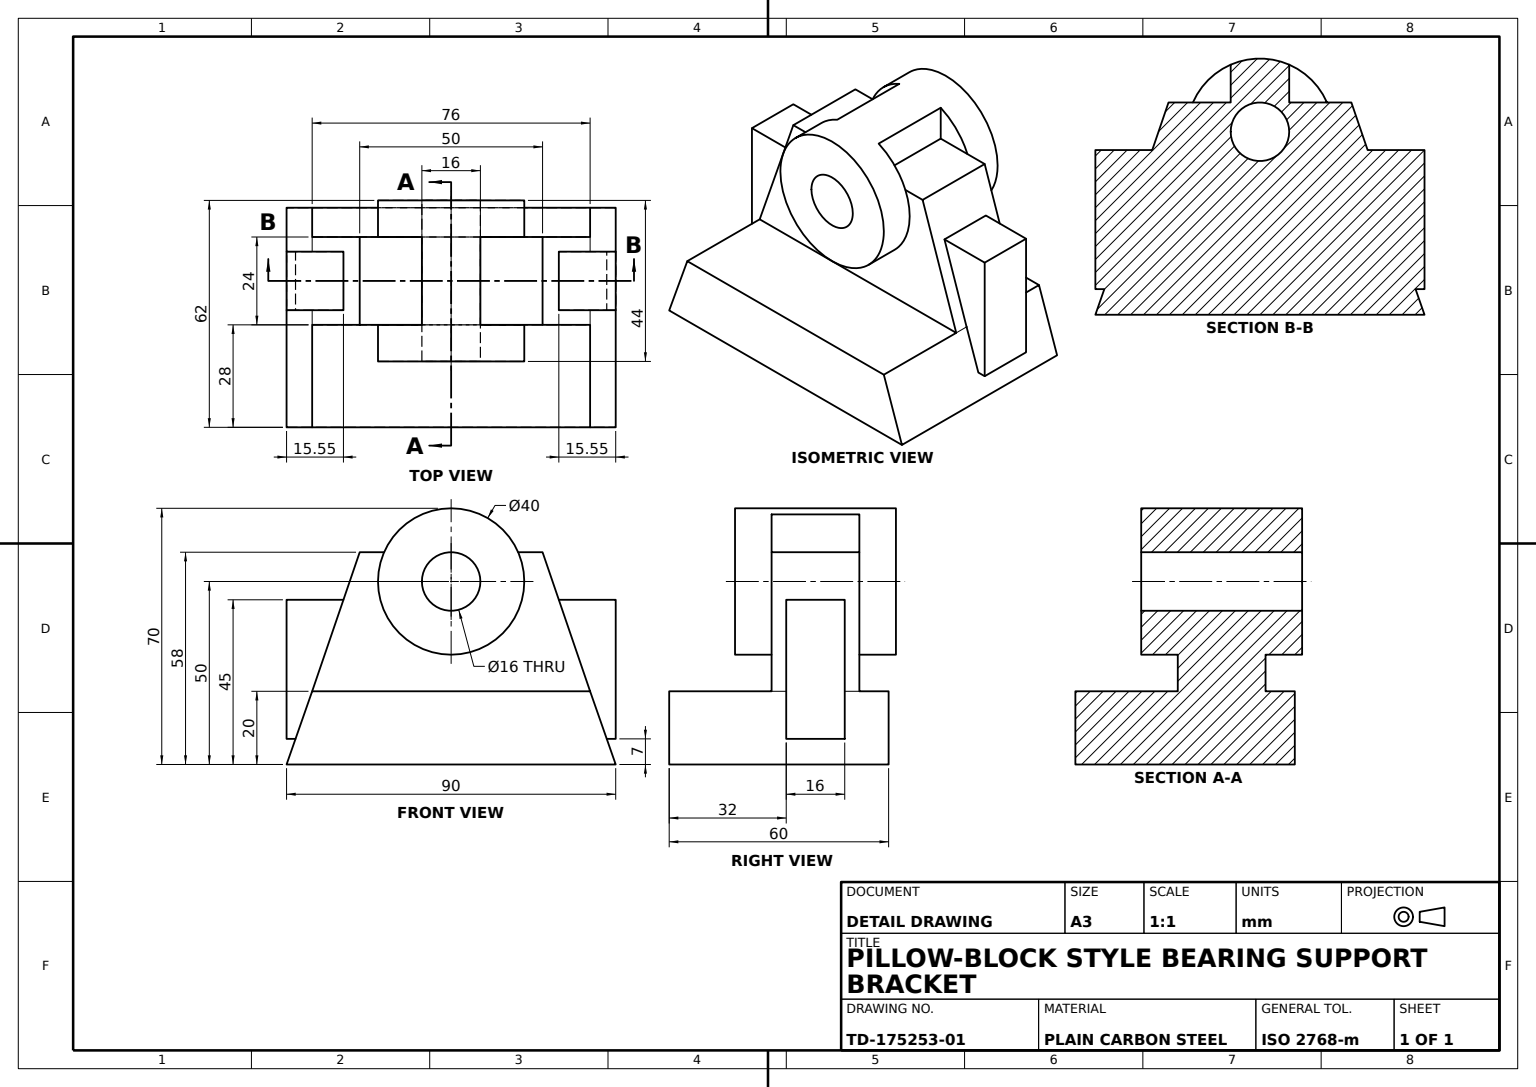
from build123d import *

# Parameters (mm, degrees)
BASE_BLOCK_DEPTH      = 20
BASE_RECESS_CUT_DEPTH = 75
HUB_CIRCLE_SKETCH_R   = 20
BEARING_HUB_DEPTH     = 44
SUPPORT_WEB_DEPTH     = 24
SIDE_WINDOW_CUT_DEPTH = 24
BEARING_BORE_SKETCH_R = 8
BEARING_BORE_DEPTH    = 57
SIDE_RIB_DEPTH        = 20


with BuildPart() as part:
    # Base Profile Sketch → Base Block (new body)
    with BuildSketch(Plane(origin=(0, 0, 0), x_dir=(1, 0, 0), z_dir=(0, 1, 0))):
        Polygon((30, 0), (30, 45), (-30, 45), (-30, -45), (30, -45), align=None)
    extrude(amount=BASE_BLOCK_DEPTH)

    # Base Recess Sketch → Base Recess Cut (cut)
    with BuildSketch(Plane(origin=(30, 0, 0), x_dir=(0, 0, -1), z_dir=(1, 0, 0))):
        Polygon((38, 20), (45, 0), (45, 20), align=None)
        Polygon((-38, 20), (-45, 0), (-45, 20), align=None)
    extrude(amount=-BASE_RECESS_CUT_DEPTH, mode=Mode.SUBTRACT)



with BuildPart() as body_2:
    # Hub Circle Sketch → Bearing Hub (new body)
    with BuildSketch(Plane(origin=(12, 0, 0), x_dir=(0, 0, -1), z_dir=(1, 0, 0))):
        with Locations((0, 50)):
            Circle(HUB_CIRCLE_SKETCH_R)
    extrude(amount=-BEARING_HUB_DEPTH)


with BuildPart() as part_1:
    add(part.part)

    add(body_2.part)  # Support Web merges body 2
    # Support Web Sketch → Support Web (add)
    with BuildSketch(Plane(origin=(2, 0, 0), x_dir=(0, 0, -1), z_dir=(1, 0, 0))):
        with BuildLine():
            Line((25, 20), (-25, 20))
            Line((-25, 20), (-38, 20))
            Line((-38, 20), (-25, 58))
            Line((-25, 58), (-18.33030278, 58))
            ThreePointArc((-18.33030278, 58), (0, 30), (18.33030278, 58))
            Line((18.33030278, 58), (25, 58))
            Line((25, 58), (38, 20))
            Line((38, 20), (25, 20))
        make_face()
    extrude(amount=-SUPPORT_WEB_DEPTH)

    # Side Window Sketch → Side Window Cut (cut)
    with BuildSketch(Plane(origin=(2, 0, 0), x_dir=(0, 0, -1), z_dir=(1, 0, 0))):
        with BuildLine():
            Line((-8, 68.33030278), (-8, 58))
            Line((-8, 58), (-18.33030278, 58))
            ThreePointArc((-18.33030278, 58), (-14.142135624, 64.142135624), (-8, 68.33030278))
        make_face()
    side_window_cut = extrude(amount=-SIDE_WINDOW_CUT_DEPTH, mode=Mode.SUBTRACT)

    # Side Window Mirror: Side Window Cut across plane
    add(side_window_cut.mirror(Plane.XY), mode=Mode.SUBTRACT)

    # Bearing Bore Sketch → Bearing Bore (cut)
    with BuildSketch(Plane(origin=(12, 0, 0), x_dir=(0, 0, -1), z_dir=(1, 0, 0))):
        with Locations((0, 50)):
            Circle(BEARING_BORE_SKETCH_R)
    extrude(amount=-BEARING_BORE_DEPTH, mode=Mode.SUBTRACT)

    # Side Rib Sketch → Side Rib (add)
    with BuildSketch(Plane.XY.offset(45)):
        Polygon((-10, 7), (-2, 7), (-2, 45), (-18, 45), (-18, 7), align=None)
    side_rib = extrude(amount=-SIDE_RIB_DEPTH)

    # Side Rib Mirror: Side Rib across plane
    add(side_rib.mirror(Plane.XY))


solid = part_1.part
